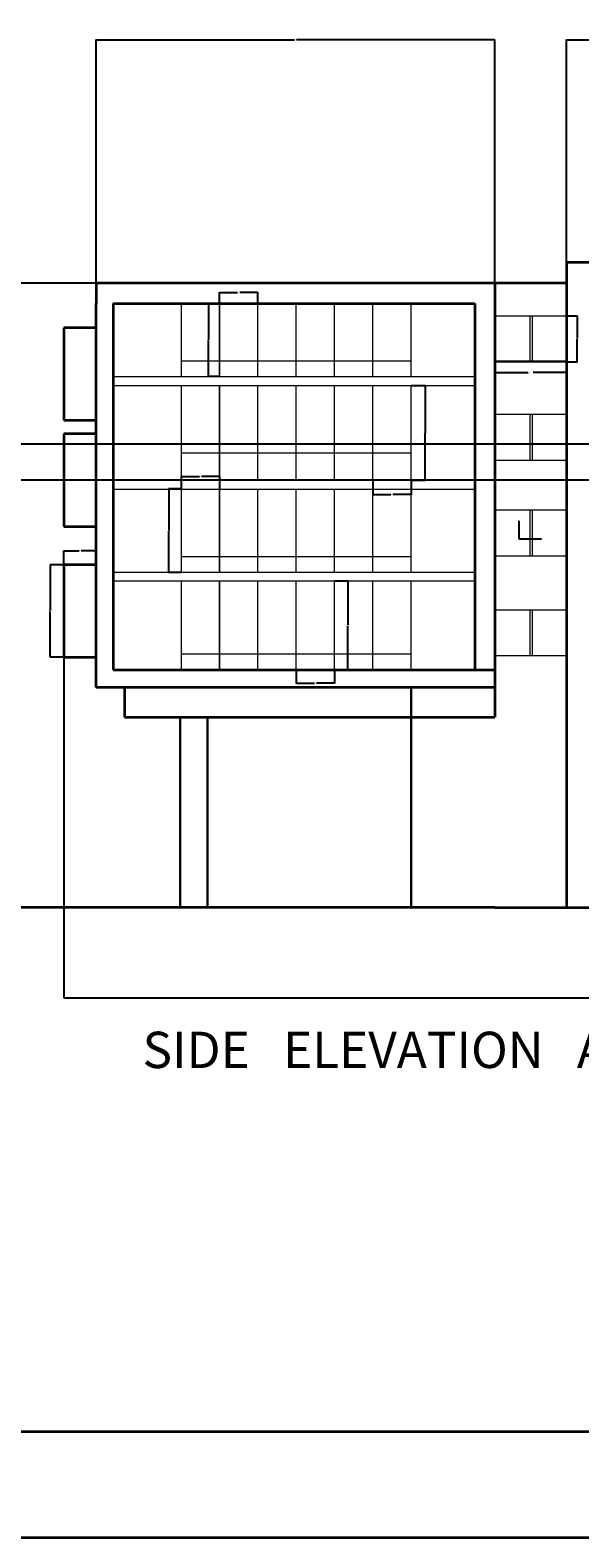
# Model space of a CAD drawing. Units: inches. Extents: x -934 to 898, y -1502 to 444.
# Tile 2 of 10: x -524 to -246, y -1502 to -739. Entities that reach past the tile are written whole.
import ezdxf

# ---------------------------------------------------------------- set-up
doc = ezdxf.new("R2010")
doc.units = ezdxf.units.IN
doc.header["$MEASUREMENT"] = 0
for name, color, linetype, lineweight in [('A-ANNO-DIMS', 2, 'Continuous', 18), ('A-ANNO-TITL', 7, 'Continuous', 30), ('A-ANNO-TTLB', 7, 'Continuous', 35), ('A-COLS', 1, 'Continuous', 30), ('A-ELEV', 7, 'Continuous', 35), ('A-GLAZ', 4, 'Continuous', 13), ('L-GRND', 7, 'Continuous', 35), ('M-HVAC', 6, 'Continuous', 25)]:
    doc.layers.add(name, color=color, linetype=linetype, lineweight=lineweight)
doc.styles.get("Standard").update_dxf_attribs({"font": 'arial.ttf'})
doc.dimstyles.get("Standard").update_dxf_attribs({"dimtxt": 0.18, "dimasz": 0.18, "dimexe": 0.18, "dimexo": 0.0625, "dimgap": 0.09, "dimtad": 0, "dimtih": 1, "dimtoh": 1, "dimdec": 4, "dimzin": 0, "dimdsep": 46, "dimtxsty": 'Standard', "dimcen": 0.09, "dimadec": 0, "dimazin": 0, "dimtfac": 1, "dimtdec": 4, "dimtofl": 0, "dimtmove": 0, "dimatfit": 3, "dimfxl": 1, "dimtolj": 1, "dimtzin": 0, "dimarcsym": 0})

# ---------------------------------------------------------------- blocks, each defined once
blk = doc.blocks.new('GLAZ-SIDE-BAY-4')
for p, q in [((0, 0), (0, 36.96)), ((19.38, 0), (19.38, 36.96)), ((0, 8.06), (19.38, 8.06))]:
    blk.add_line(p, q)
blk = doc.blocks.new('GLAZ-SIDE-BAY-3')
for p, q in [((0, 0), (0, 47.94)), ((19.38, 0), (19.38, 47.94)), ((0, 13.9), (19.38, 13.9))]:
    blk.add_line(p, q)
blk = doc.blocks.new('GLAZ-SIDE-BAY-2')
for p, q in [((0, 0), (0, 42.17)), ((19.38, 0), (19.38, 42.17)), ((0, 8.06), (19.38, 8.06))]:
    blk.add_line(p, q)
blk = doc.blocks.new('GLAZ-SIDE-BAY-1')
for p, q in [((0, 0), (0, 44.87)), ((19.38, 0), (19.38, 44.87)), ((0, 8.06), (19.38, 8.06))]:
    blk.add_line(p, q)
blk = doc.blocks.new('FACADE-PROJECTION-TALL')
for p, q in [((16.35, 46.75), (0, 46.75)), ((0, 46.75), (0, 0)), ((0, 0), (16.35, 0))]:
    blk.add_line(p, q)
blk = doc.blocks.new('CORE-CONNECTOR-BAY')
for p, q in [((0, 23.2), (36.28, 23.2)), ((17.63, 23.2), (17.63, 0)), ((18.87, 23.2), (18.87, 0)), ((0, 0), (36.28, 0))]:
    blk.add_line(p, q)
blk = doc.blocks.new('*D59')
at = {"layer": 'A-ANNO-DIMS', "color": 0, "lineweight": -2, "transparency": 16777216}
for p, q in [((-428.25, -877.63), (-433.91, -877.63)), ((-433.73, -877.81), (-433.73, -895.93)), ((-433.73, -914.41), (-433.73, -896.29)), ((-428.25, -914.59), (-433.91, -914.59))]:
    blk.add_line(p, q, dxfattribs=at)
at = {"layer": 'A-ANNO-DIMS', "color": 0, "transparency": 16777216}
for points in [[(-433.76, -877.81), (-433.7, -877.81), (-433.73, -877.63)], [(-433.76, -914.41), (-433.7, -914.41), (-433.73, -914.59)]]:
    blk.add_solid(points, dxfattribs=at)
at = {"layer": 'Defpoints', "color": 0, "transparency": 16777216}
for p in [(-433.73, -877.63), (-428.19, -877.63), (-428.19, -914.59)]:
    blk.add_point(p, dxfattribs=at)
at = {"layer": 'A-ANNO-DIMS', "color": 0, "transparency": 16777216, "insert": (-433.73, -896.11), "char_height": 0.18, "attachment_point": 5}
blk.add_mtext('\\A1;BAY 4 37 TYP.', dxfattribs=at)
blk = doc.blocks.new('*D60')
at = {"layer": 'A-ANNO-DIMS', "color": 0, "lineweight": -2, "transparency": 16777216}
for p, q in [((-428.19, -877.56), (-428.19, -871.9)), ((-428.01, -872.08), (-419.02, -872.08)), ((-408.99, -872.08), (-417.98, -872.08)), ((-408.81, -877.56), (-408.81, -871.9))]:
    blk.add_line(p, q, dxfattribs=at)
at = {"layer": 'A-ANNO-DIMS', "color": 0, "transparency": 16777216}
for points in [[(-428.01, -872.05), (-428.01, -872.11), (-428.19, -872.08)], [(-408.99, -872.05), (-408.99, -872.11), (-408.81, -872.08)]]:
    blk.add_solid(points, dxfattribs=at)
at = {"layer": 'Defpoints', "color": 0, "transparency": 16777216}
for p in [(-408.81, -872.08), (-428.19, -877.63), (-408.81, -877.63)]:
    blk.add_point(p, dxfattribs=at)
at = {"layer": 'A-ANNO-DIMS', "color": 0, "transparency": 16777216, "insert": (-418.5, -872.08), "char_height": 0.18, "attachment_point": 5}
blk.add_mtext('\\A1;19 TYP.', dxfattribs=at)
blk = doc.blocks.new('*D61')
at = {"layer": 'A-ANNO-DIMS', "color": 0, "lineweight": -2, "transparency": 16777216}
for p, q in [((-331.28, -919.02), (-323.97, -919.02)), ((-324.15, -919.2), (-324.15, -942.8)), ((-324.15, -966.78), (-324.15, -943.17)), ((-331.28, -966.96), (-323.97, -966.96))]:
    blk.add_line(p, q, dxfattribs=at)
at = {"layer": 'A-ANNO-DIMS', "color": 0, "transparency": 16777216}
for points in [[(-324.18, -919.2), (-324.12, -919.2), (-324.15, -919.02)], [(-324.18, -966.78), (-324.12, -966.78), (-324.15, -966.96)]]:
    blk.add_solid(points, dxfattribs=at)
at = {"layer": 'Defpoints', "color": 0, "transparency": 16777216}
for p in [(-331.35, -919.02), (-324.15, -919.02), (-331.35, -966.96)]:
    blk.add_point(p, dxfattribs=at)
at = {"layer": 'A-ANNO-DIMS', "color": 0, "transparency": 16777216, "insert": (-324.15, -942.99), "char_height": 0.18, "attachment_point": 5}
blk.add_mtext('\\A1;BAY 3 48 TYP.', dxfattribs=at)
blk = doc.blocks.new('*D62')
at = {"layer": 'A-ANNO-DIMS', "color": 0, "lineweight": -2, "transparency": 16777216}
for p, q in [((-350.73, -967.02), (-350.73, -974.33)), ((-331.35, -967.02), (-331.35, -974.33)), ((-350.55, -974.15), (-341.56, -974.15)), ((-331.53, -974.15), (-340.52, -974.15))]:
    blk.add_line(p, q, dxfattribs=at)
at = {"layer": 'A-ANNO-DIMS', "color": 0, "transparency": 16777216}
for points in [[(-350.55, -974.12), (-350.55, -974.18), (-350.73, -974.15)], [(-331.53, -974.12), (-331.53, -974.18), (-331.35, -974.15)]]:
    blk.add_solid(points, dxfattribs=at)
at = {"layer": 'Defpoints', "color": 0, "transparency": 16777216}
for p in [(-350.73, -966.96), (-331.35, -966.96), (-331.35, -974.15)]:
    blk.add_point(p, dxfattribs=at)
at = {"layer": 'A-ANNO-DIMS', "color": 0, "transparency": 16777216, "insert": (-341.04, -974.15), "char_height": 0.18, "attachment_point": 5}
blk.add_mtext('\\A1;19 TYP.', dxfattribs=at)
blk = doc.blocks.new('*D63')
at = {"layer": 'A-ANNO-DIMS', "color": 0, "lineweight": -2, "transparency": 16777216}
for p, q in [((-447.54, -971.38), (-453.99, -971.38)), ((-453.81, -971.56), (-453.81, -992.29)), ((-453.81, -1013.38), (-453.81, -992.65)), ((-447.54, -1013.56), (-453.99, -1013.56))]:
    blk.add_line(p, q, dxfattribs=at)
at = {"layer": 'A-ANNO-DIMS', "color": 0, "transparency": 16777216}
for points in [[(-453.84, -971.56), (-453.78, -971.56), (-453.81, -971.38)], [(-453.84, -1013.38), (-453.78, -1013.38), (-453.81, -1013.56)]]:
    blk.add_solid(points, dxfattribs=at)
at = {"layer": 'Defpoints', "color": 0, "transparency": 16777216}
for p in [(-453.81, -971.38), (-447.48, -971.38), (-447.48, -1013.56)]:
    blk.add_point(p, dxfattribs=at)
at = {"layer": 'A-ANNO-DIMS', "color": 0, "transparency": 16777216, "insert": (-453.81, -992.47), "char_height": 0.18, "attachment_point": 5}
blk.add_mtext('\\A1;BAY 2 42 TYP.', dxfattribs=at)
blk = doc.blocks.new('*D64')
at = {"layer": 'A-ANNO-DIMS', "color": 0, "lineweight": -2, "transparency": 16777216}
for p, q in [((-447.48, -971.32), (-447.48, -964.88)), ((-447.3, -965.06), (-438.31, -965.06)), ((-428.28, -965.06), (-437.27, -965.06)), ((-428.1, -971.32), (-428.1, -964.88))]:
    blk.add_line(p, q, dxfattribs=at)
at = {"layer": 'A-ANNO-DIMS', "color": 0, "transparency": 16777216}
for points in [[(-447.3, -965.03), (-447.3, -965.09), (-447.48, -965.06)], [(-428.28, -965.03), (-428.28, -965.09), (-428.1, -965.06)]]:
    blk.add_solid(points, dxfattribs=at)
at = {"layer": 'Defpoints', "color": 0, "transparency": 16777216}
for p in [(-428.1, -965.06), (-447.48, -971.38), (-428.1, -971.38)]:
    blk.add_point(p, dxfattribs=at)
at = {"layer": 'A-ANNO-DIMS', "color": 0, "transparency": 16777216, "insert": (-437.79, -965.06), "char_height": 0.18, "attachment_point": 5}
blk.add_mtext('\\A1;19 TYP.', dxfattribs=at)
blk = doc.blocks.new('*D65')
at = {"layer": 'A-ANNO-DIMS', "color": 0, "lineweight": -2, "transparency": 16777216}
for p, q in [((-369.95, -1017.85), (-363.1, -1017.85)), ((-363.28, -1018.03), (-363.28, -1040.1)), ((-363.28, -1062.54), (-363.28, -1040.47)), ((-369.95, -1062.72), (-363.1, -1062.72))]:
    blk.add_line(p, q, dxfattribs=at)
at = {"layer": 'A-ANNO-DIMS', "color": 0, "transparency": 16777216}
for points in [[(-363.31, -1018.03), (-363.25, -1018.03), (-363.28, -1017.85)], [(-363.31, -1062.54), (-363.25, -1062.54), (-363.28, -1062.72)]]:
    blk.add_solid(points, dxfattribs=at)
at = {"layer": 'Defpoints', "color": 0, "transparency": 16777216}
for p in [(-370.01, -1017.85), (-363.28, -1017.85), (-370.01, -1062.72)]:
    blk.add_point(p, dxfattribs=at)
at = {"layer": 'A-ANNO-DIMS', "color": 0, "transparency": 16777216, "insert": (-363.28, -1040.28), "char_height": 0.18, "attachment_point": 5}
blk.add_mtext('\\A1;BAY 1 45 TYP.', dxfattribs=at)
blk = doc.blocks.new('*D66')
at = {"layer": 'A-ANNO-DIMS', "color": 0, "lineweight": -2, "transparency": 16777216}
for p, q in [((-389.39, -1062.78), (-389.39, -1069.63)), ((-370.01, -1062.78), (-370.01, -1069.63)), ((-389.21, -1069.45), (-380.22, -1069.45)), ((-370.19, -1069.45), (-379.18, -1069.45))]:
    blk.add_line(p, q, dxfattribs=at)
at = {"layer": 'A-ANNO-DIMS', "color": 0, "transparency": 16777216}
for points in [[(-389.21, -1069.42), (-389.21, -1069.48), (-389.39, -1069.45)], [(-370.19, -1069.42), (-370.19, -1069.48), (-370.01, -1069.45)]]:
    blk.add_solid(points, dxfattribs=at)
at = {"layer": 'Defpoints', "color": 0, "transparency": 16777216}
for p in [(-389.39, -1062.72), (-370.01, -1062.72), (-370.01, -1069.45)]:
    blk.add_point(p, dxfattribs=at)
at = {"layer": 'A-ANNO-DIMS', "color": 0, "transparency": 16777216, "insert": (-379.7, -1069.45), "char_height": 0.18, "attachment_point": 5}
blk.add_mtext('\\A1;19 TYP.', dxfattribs=at)
blk = doc.blocks.new('*D69')
at = {"layer": 'A-ANNO-DIMS', "color": 0, "lineweight": -2, "transparency": 16777216}
for p, q in [((-288.98, -907.15), (-288.98, -912.71)), ((-288.8, -912.53), (-272.08, -912.53)), ((-252.88, -912.53), (-269.6, -912.53)), ((-252.7, -907.15), (-252.7, -912.71))]:
    blk.add_line(p, q, dxfattribs=at)
at = {"layer": 'A-ANNO-DIMS', "color": 0, "transparency": 16777216}
for points in [[(-288.8, -912.5), (-288.8, -912.56), (-288.98, -912.53)], [(-252.88, -912.5), (-252.88, -912.56), (-252.7, -912.53)]]:
    blk.add_solid(points, dxfattribs=at)
at = {"layer": 'Defpoints', "color": 0, "transparency": 16777216}
for p in [(-288.98, -907.09), (-252.7, -907.09), (-252.7, -912.53)]:
    blk.add_point(p, dxfattribs=at)
at = {"layer": 'A-ANNO-DIMS', "color": 0, "transparency": 16777216, "insert": (-270.84, -912.53), "char_height": 0.18, "attachment_point": 5}
blk.add_mtext('\\A1;CORE LINK 36 TYP.', dxfattribs=at)
blk = doc.blocks.new('*D70')
at = {"layer": 'A-ANNO-DIMS', "color": 0, "lineweight": -2, "transparency": 16777216}
for p, q in [((-252.64, -883.88), (-247.08, -883.88)), ((-247.26, -884.06), (-247.26, -895.3)), ((-247.26, -906.91), (-247.26, -895.67)), ((-252.64, -907.09), (-247.08, -907.09))]:
    blk.add_line(p, q, dxfattribs=at)
at = {"layer": 'A-ANNO-DIMS', "color": 0, "transparency": 16777216}
for points in [[(-247.29, -884.06), (-247.23, -884.06), (-247.26, -883.88)], [(-247.29, -906.91), (-247.23, -906.91), (-247.26, -907.09)]]:
    blk.add_solid(points, dxfattribs=at)
at = {"layer": 'Defpoints', "color": 0, "transparency": 16777216}
for p in [(-252.7, -883.88), (-247.26, -883.88), (-252.7, -907.09)]:
    blk.add_point(p, dxfattribs=at)
at = {"layer": 'A-ANNO-DIMS', "color": 0, "transparency": 16777216, "insert": (-247.26, -895.49), "char_height": 0.18, "attachment_point": 5}
blk.add_mtext('\\A1;23 TYP.', dxfattribs=at)
blk = doc.blocks.new('*D71')
at = {"layer": 'A-ANNO-DIMS', "color": 0, "lineweight": -2, "transparency": 16777216}
for p, q in [((-506.93, -1009.67), (-514.06, -1009.67)), ((-513.88, -1009.85), (-513.88, -1032.87)), ((-513.88, -1056.25), (-513.88, -1033.23)), ((-506.93, -1056.43), (-514.06, -1056.43))]:
    blk.add_line(p, q, dxfattribs=at)
at = {"layer": 'A-ANNO-DIMS', "color": 0, "transparency": 16777216}
for points in [[(-513.91, -1009.85), (-513.85, -1009.85), (-513.88, -1009.67)], [(-513.91, -1056.25), (-513.85, -1056.25), (-513.88, -1056.43)]]:
    blk.add_solid(points, dxfattribs=at)
at = {"layer": 'Defpoints', "color": 0, "transparency": 16777216}
for p in [(-513.88, -1009.67), (-506.87, -1009.67), (-506.87, -1056.43)]:
    blk.add_point(p, dxfattribs=at)
at = {"layer": 'A-ANNO-DIMS', "color": 0, "transparency": 16777216, "insert": (-513.88, -1033.05), "char_height": 0.18, "attachment_point": 5}
blk.add_mtext('\\A1;FACADE FIN 47 TYP.', dxfattribs=at)
blk = doc.blocks.new('*D72')
at = {"layer": 'A-ANNO-DIMS', "color": 0, "lineweight": -2, "transparency": 16777216}
for p, q in [((-506.87, -1009.61), (-506.87, -1002.48)), ((-506.69, -1002.66), (-499.21, -1002.66)), ((-490.7, -1002.66), (-498.18, -1002.66)), ((-490.52, -1009.61), (-490.52, -1002.48))]:
    blk.add_line(p, q, dxfattribs=at)
at = {"layer": 'A-ANNO-DIMS', "color": 0, "transparency": 16777216}
for points in [[(-506.69, -1002.63), (-506.69, -1002.69), (-506.87, -1002.66)], [(-490.7, -1002.63), (-490.7, -1002.69), (-490.52, -1002.66)]]:
    blk.add_solid(points, dxfattribs=at)
at = {"layer": 'Defpoints', "color": 0, "transparency": 16777216}
for p in [(-490.52, -1002.66), (-506.87, -1009.67), (-490.52, -1009.67)]:
    blk.add_point(p, dxfattribs=at)
at = {"layer": 'A-ANNO-DIMS', "color": 0, "transparency": 16777216, "insert": (-498.7, -1002.66), "char_height": 0.18, "attachment_point": 5}
blk.add_mtext('\\A1;16 TYP.', dxfattribs=at)
blk = doc.blocks.new('*D107')
at = {"layer": 'A-ANNO-DIMS', "color": 0, "lineweight": -2, "transparency": 16777216}
for p, q in [((-506.87, -1056.49), (-506.87, -1228.82)), ((249.98, -1183.07), (249.98, -1228.82)), ((-506.69, -1228.64), (-128.84, -1228.64)), ((249.8, -1228.64), (-128.05, -1228.64))]:
    blk.add_line(p, q, dxfattribs=at)
at = {"layer": 'A-ANNO-DIMS', "color": 0, "transparency": 16777216}
for points in [[(-506.69, -1228.61), (-506.69, -1228.67), (-506.87, -1228.64)], [(249.8, -1228.61), (249.8, -1228.67), (249.98, -1228.64)]]:
    blk.add_solid(points, dxfattribs=at)
at = {"layer": 'Defpoints', "color": 0, "transparency": 16777216}
for p in [(-506.87, -1056.43), (249.98, -1183.01), (249.98, -1228.64)]:
    blk.add_point(p, dxfattribs=at)
at = {"layer": 'A-ANNO-DIMS', "color": 0, "transparency": 16777216, "insert": (-128.45, -1228.64), "char_height": 0.18, "attachment_point": 5}
blk.add_mtext('\\A1;756.8', dxfattribs=at)
blk = doc.blocks.new('*D109')
at = {"layer": 'A-ANNO-DIMS', "color": 0, "lineweight": -2, "transparency": 16777216}
for p, q in [((-490.52, -867.28), (-490.52, -744.15)), ((-490.34, -744.33), (-390.21, -744.33)), ((-289.16, -744.33), (-389.29, -744.33)), ((-288.98, -867.28), (-288.98, -744.15))]:
    blk.add_line(p, q, dxfattribs=at)
at = {"layer": 'A-ANNO-DIMS', "color": 0, "transparency": 16777216}
for points in [[(-490.34, -744.3), (-490.34, -744.36), (-490.52, -744.33)], [(-289.16, -744.3), (-289.16, -744.36), (-288.98, -744.33)]]:
    blk.add_solid(points, dxfattribs=at)
at = {"layer": 'Defpoints', "color": 0, "transparency": 16777216}
for p in [(-288.98, -744.33), (-490.52, -867.34), (-288.98, -867.34)]:
    blk.add_point(p, dxfattribs=at)
at = {"layer": 'A-ANNO-DIMS', "color": 0, "transparency": 16777216, "insert": (-389.75, -744.33), "char_height": 0.18, "attachment_point": 5}
blk.add_mtext('\\A1;201.54', dxfattribs=at)
blk = doc.blocks.new('*D110')
at = {"layer": 'A-ANNO-DIMS', "color": 0, "lineweight": -2, "transparency": 16777216}
for p, q in [((-252.7, -856.85), (-252.7, -744.15)), ((-252.52, -744.33), (-213.38, -744.33)), ((-173.45, -744.33), (-212.59, -744.33)), ((-173.27, -856.85), (-173.27, -744.15))]:
    blk.add_line(p, q, dxfattribs=at)
at = {"layer": 'A-ANNO-DIMS', "color": 0, "transparency": 16777216}
for points in [[(-252.52, -744.3), (-252.52, -744.36), (-252.7, -744.33)], [(-173.45, -744.3), (-173.45, -744.36), (-173.27, -744.33)]]:
    blk.add_solid(points, dxfattribs=at)
at = {"layer": 'Defpoints', "color": 0, "transparency": 16777216}
for p in [(-173.27, -744.33), (-252.7, -856.91), (-173.27, -856.91)]:
    blk.add_point(p, dxfattribs=at)
at = {"layer": 'A-ANNO-DIMS', "color": 0, "transparency": 16777216, "insert": (-212.98, -744.33), "char_height": 0.18, "attachment_point": 5}
blk.add_mtext('\\A1;79.43', dxfattribs=at)
blk = doc.blocks.new('*D114')
at = {"layer": 'A-ANNO-DIMS', "color": 0, "lineweight": -2, "transparency": 16777216}
for p, q in [((-122.37, -948.66), (-637.55, -948.66)), ((-637.37, -948.84), (-637.37, -957.63)), ((-637.37, -966.78), (-637.37, -957.99)), ((-142.26, -966.96), (-637.55, -966.96))]:
    blk.add_line(p, q, dxfattribs=at)
at = {"layer": 'A-ANNO-DIMS', "color": 0, "transparency": 16777216}
for points in [[(-637.4, -948.84), (-637.34, -948.84), (-637.37, -948.66)], [(-637.4, -966.78), (-637.34, -966.78), (-637.37, -966.96)]]:
    blk.add_solid(points, dxfattribs=at)
at = {"layer": 'Defpoints', "color": 0, "transparency": 16777216}
for p in [(-637.37, -948.66), (-122.31, -948.66), (-142.19, -966.96)]:
    blk.add_point(p, dxfattribs=at)
at = {"layer": 'A-ANNO-DIMS', "color": 0, "transparency": 16777216, "insert": (-637.37, -957.81), "char_height": 0.18, "attachment_point": 5}
blk.add_mtext('\\A1;18.294', dxfattribs=at)
blk = doc.blocks.new('*D117')
at = {"layer": 'A-ANNO-DIMS', "color": 0, "lineweight": -2, "transparency": 16777216}
for p, q in [((-490.58, -867.34), (-637.55, -867.34)), ((-637.37, -867.52), (-637.37, -1024.99)), ((-637.37, -1182.83), (-637.37, -1025.36)), ((-448.1, -1183.01), (-637.55, -1183.01))]:
    blk.add_line(p, q, dxfattribs=at)
at = {"layer": 'A-ANNO-DIMS', "color": 0, "transparency": 16777216}
for points in [[(-637.4, -867.52), (-637.34, -867.52), (-637.37, -867.34)], [(-637.4, -1182.83), (-637.34, -1182.83), (-637.37, -1183.01)]]:
    blk.add_solid(points, dxfattribs=at)
at = {"layer": 'Defpoints', "color": 0, "transparency": 16777216}
for p in [(-637.37, -867.34), (-490.52, -867.34), (-448.04, -1183.01)]:
    blk.add_point(p, dxfattribs=at)
at = {"layer": 'A-ANNO-DIMS', "color": 0, "transparency": 16777216, "insert": (-637.37, -1025.17), "char_height": 0.18, "attachment_point": 5}
blk.add_mtext('\\A1;315.7', dxfattribs=at)

msp = doc.modelspace()

# ---------------------------------------------------------------- linework, layer by layer
at = {"layer": 'A-ANNO-TTLB'}
for points in [[(-933.5092, 444.4646), (897.7239, 444.4646), (897.7239, -1501.5858), (-933.5092, -1501.5858)], [(-892.081, 380.0228), (832.9871, 380.0228), (832.9871, -1448.0237), (-892.081, -1448.0237)]]:
    msp.add_lwpolyline(points, close=True, dxfattribs=at)
at = {"layer": 'A-COLS'}
for p, q in [((-331.3451, -1086.7702), (-331.3451, -1071.6451)), ((-448.0415, -1086.7702), (-448.0415, -1183.0104)), ((-434.2287, -1086.7702), (-434.2287, -1183.0104)), ((-331.3451, -1086.7702), (-331.3451, -1183.0104))]:
    msp.add_line(p, q, dxfattribs=at)
at = {"layer": 'A-ELEV'}
for p, q in [((-173.2689, -856.9131), (-252.6991, -856.9131)), ((-252.6991, -856.9131), (-252.6991, -867.3393)), ((-481.9907, -867.3393), (-490.5224, -867.3393)), ((-490.5224, -867.3393), (-490.5224, -877.626)), ((-252.6991, -867.3393), (-481.9907, -867.3393)), ((-288.9776, -867.3393), (-288.9776, -1062.7319)), ((-252.6991, -867.3393), (-252.6991, -1062.7319)), ((-490.5224, -1071.6451), (-490.5224, -877.626)), ((-481.9907, -877.626), (-481.9907, -1062.7319)), ((-481.9907, -877.626), (-299.1015, -877.626)), ((-299.1015, -877.626), (-299.1015, -1062.7319)), ((-481.9907, -1062.7319), (-299.1015, -1062.7319)), ((-299.1015, -1062.7319), (-288.9776, -1062.7319)), ((-288.9776, -1062.7319), (-288.9776, -1086.7702)), ((-252.6991, -1062.7319), (-252.6991, -1183.0104)), ((-288.9776, -1071.6451), (-490.5224, -1071.6451)), ((-476.149, -1071.6451), (-476.149, -1086.7702)), ((-476.149, -1086.7702), (-288.9776, -1086.7702))]:
    msp.add_line(p, q, dxfattribs=at)
at = {"layer": 'A-GLAZ'}
for p, q in [((-481.9907, -877.626), (-299.1015, -877.626)), ((-288.9776, -906.532), (-252.6991, -906.532)), ((-481.9907, -914.5889), (-299.1015, -914.5889)), ((-481.9907, -919.0154), (-299.1015, -919.0154)), ((-481.9907, -966.9581), (-299.1015, -966.9581)), ((-331.3451, -966.9581), (-299.1015, -966.9581)), ((-481.9907, -971.3846), (-299.1015, -971.3846)), ((-481.9907, -1013.4232), (-299.1015, -1013.4232)), ((-481.9907, -1017.8497), (-299.1015, -1017.8497)), ((-331.3451, -1062.7171), (-331.3451, -1062.7319))]:
    msp.add_line(p, q, dxfattribs=at)
at = {"layer": 'L-GRND'}
for q in [(-591.8658, -1183.0104), (308.1933, -1183.0104)]:
    msp.add_line((-288.9776, -1183.0104), q, dxfattribs=at)
at = {"layer": 'M-HVAC'}
for p, q in [((-276.854, -987.4652), (-276.854, -996.493)), ((-276.854, -996.493), (-265.3047, -996.493))]:
    msp.add_line(p, q, dxfattribs=at)

# ---------------------------------------------------------------- block references
at = {"layer": 'A-ELEV'}
for p in [(-506.8678, -936.6058), (-506.8678, -990.2794), (-506.8678, -1056.4266)]:
    msp.add_blockref('FACADE-PROJECTION-TALL', p, dxfattribs=at)
at = {"layer": 'A-GLAZ'}
for name, p in [('GLAZ-SIDE-BAY-4', (-447.4808, -914.5889)), ('GLAZ-SIDE-BAY-4', (-428.1859, -914.5889)), ('GLAZ-SIDE-BAY-4', (-408.8696, -914.5889)), ('GLAZ-SIDE-BAY-4', (-389.3942, -914.5889)), ('GLAZ-SIDE-BAY-4', (-370.0872, -914.5889)), ('GLAZ-SIDE-BAY-4', (-350.726, -914.5889)), ('CORE-CONNECTOR-BAY', (-288.9776, -907.0873)), ('GLAZ-SIDE-BAY-3', (-447.4808, -966.9581)), ('GLAZ-SIDE-BAY-3', (-428.1859, -966.9581)), ('GLAZ-SIDE-BAY-3', (-408.8696, -966.9581)), ('GLAZ-SIDE-BAY-3', (-389.3942, -966.9581)), ('GLAZ-SIDE-BAY-3', (-370.0872, -966.9581)), ('GLAZ-SIDE-BAY-3', (-350.726, -966.9581)), ('CORE-CONNECTOR-BAY', (-288.9776, -956.7866)), ('GLAZ-SIDE-BAY-2', (-447.4808, -1013.5581)), ('GLAZ-SIDE-BAY-2', (-428.1859, -1013.5581)), ('GLAZ-SIDE-BAY-2', (-408.8696, -1013.5581)), ('GLAZ-SIDE-BAY-2', (-389.3942, -1013.5581)), ('GLAZ-SIDE-BAY-2', (-370.0872, -1013.5581)), ('GLAZ-SIDE-BAY-2', (-350.726, -1013.5581)), ('CORE-CONNECTOR-BAY', (-288.9776, -1005.1879)), ('GLAZ-SIDE-BAY-1', (-447.4808, -1062.7171)), ('GLAZ-SIDE-BAY-1', (-428.1859, -1062.7171)), ('GLAZ-SIDE-BAY-1', (-408.8696, -1062.7171)), ('GLAZ-SIDE-BAY-1', (-389.3942, -1062.7171)), ('GLAZ-SIDE-BAY-1', (-370.0872, -1062.7171)), ('GLAZ-SIDE-BAY-1', (-350.726, -1062.7171)), ('CORE-CONNECTOR-BAY', (-288.9776, -1055.6296))]:
    msp.add_blockref(name, p, dxfattribs=at)

# ---------------------------------------------------------------- texts
at = {"layer": 'A-ANNO-TITL'}
msp.add_text('SIDE   ELEVATION   AND MECHNICAL   INTERTRALS', height=18.353224, dxfattribs=at).set_placement((-467.0954, -1264.0952))

# ---------------------------------------------------------------- dimensions: what is measured, and where the dimension line sits
at = {"layer": 'A-ANNO-DIMS'}
for base, p1, p2, override, picture, middle in [((-288.9776, -744.326), (-490.5224, -867.3393), (-288.9776, -867.3393), {"dimdec": 2, "dimlfac": 1, "dimrnd": 0, "dimzin": 0, "dimdsep": 46, "dimlunit": 2}, '*D109', (-389.75, -744.326)), ((-173.2689, -744.326), (-252.6991, -856.9131), (-173.2689, -856.9131), {"dimdec": 2, "dimlfac": 1, "dimrnd": 0, "dimzin": 0, "dimdsep": 46, "dimlunit": 2}, '*D110', (-212.984, -744.326)), ((249.977, -1228.6394), (-506.8678, -1056.4266), (249.977, -1183.0104), {"dimdec": 1, "dimlfac": 1, "dimrnd": 0, "dimzin": 0, "dimdsep": 46, "dimlunit": 2}, '*D107', (-128.4454, -1228.6394))]:
    dim = msp.add_linear_dim(base=base, p1=p1, p2=p2, dimstyle='Standard', override=override, dxfattribs=at)
    dim.commit()
    dim.dimension.update_dxf_attribs({"geometry": picture, "text_midpoint": middle})
for base, p1, p2, override, picture, middle in [((-637.3658, -867.3393), (-448.0415, -1183.0104), (-490.5224, -867.3393), {"dimdec": 1, "dimlfac": 1, "dimrnd": 0, "dimzin": 0, "dimdsep": 46, "dimlunit": 2}, '*D117', (-637.3658, -1025.1749)), ((-637.3658, -948.6643), (-142.1926, -966.9581), (-122.305, -948.6643), {"dimdec": 3, "dimlfac": 1, "dimrnd": 0, "dimzin": 0, "dimdsep": 46, "dimlunit": 2}, '*D114', (-637.3658, -957.8112))]:
    dim = msp.add_linear_dim(base=base, p1=p1, p2=p2, angle=90, dimstyle='Standard', override=override, dxfattribs=at)
    dim.commit()
    dim.dimension.update_dxf_attribs({"geometry": picture, "text_midpoint": middle})
for base, p1, p2, text, picture, middle in [((-408.805, -872.0815), (-428.1859, -877.626), (-408.805, -877.626), '<> TYP.', '*D60', (-418.4955, -872.0815)), ((-252.6991, -912.5291), (-288.9776, -907.0873), (-252.6991, -907.0873), 'CORE LINK <> TYP.', '*D69', (-270.8384, -912.5291)), ((-428.1, -965.0586), (-447.4808, -971.3846), (-428.1, -971.3846), '<> TYP.', '*D64', (-437.7904, -965.0586)), ((-331.3451, -974.1495), (-350.726, -966.9581), (-331.3451, -966.9581), '<> TYP.', '*D62', (-341.0355, -974.1495)), ((-490.5224, -1002.6611), (-506.8678, -1009.674), (-490.5224, -1009.674), '<> TYP.', '*D72', (-498.6951, -1002.6611)), ((-370.0133, -1069.4473), (-389.3942, -1062.7171), (-370.0133, -1062.7171), '<> TYP.', '*D66', (-379.7038, -1069.4473))]:
    dim = msp.add_linear_dim(base=base, p1=p1, p2=p2, text=text, dimstyle='Standard', override={"dimdec": 0, "dimlfac": 1, "dimrnd": 0, "dimzin": 0, "dimdsep": 46, "dimlunit": 2}, dxfattribs=at)
    dim.commit()
    dim.dimension.update_dxf_attribs({"geometry": picture, "text_midpoint": middle})
for base, p1, p2, text, picture, middle in [((-433.7303, -877.626), (-428.1859, -914.5889), (-428.1859, -877.626), 'BAY 4 <> TYP.', '*D59', (-433.7303, -896.1074)), ((-247.2573, -883.8841), (-252.6991, -907.0873), (-252.6991, -883.8841), '<> TYP.', '*D70', (-247.2573, -895.4857)), ((-324.1537, -919.0154), (-331.3451, -966.9581), (-331.3451, -919.0154), 'BAY 3 <> TYP.', '*D61', (-324.1537, -942.9867)), ((-453.8069, -971.3846), (-447.4808, -1013.5581), (-447.4808, -971.3846), 'BAY 2 <> TYP.', '*D63', (-453.8069, -992.4714)), ((-513.8807, -1009.674), (-506.8678, -1056.4266), (-506.8678, -1009.674), 'FACADE FIN <> TYP.', '*D71', (-513.8807, -1033.0503)), ((-363.2832, -1017.8497), (-370.0133, -1062.7171), (-370.0133, -1017.8497), 'BAY 1 <> TYP.', '*D65', (-363.2832, -1040.2834))]:
    dim = msp.add_linear_dim(base=base, p1=p1, p2=p2, angle=90, text=text, dimstyle='Standard', override={"dimdec": 0, "dimlfac": 1, "dimrnd": 0, "dimzin": 0, "dimdsep": 46, "dimlunit": 2}, dxfattribs=at)
    dim.commit()
    dim.dimension.update_dxf_attribs({"geometry": picture, "text_midpoint": middle})

doc.saveas('drawing.dxf')
